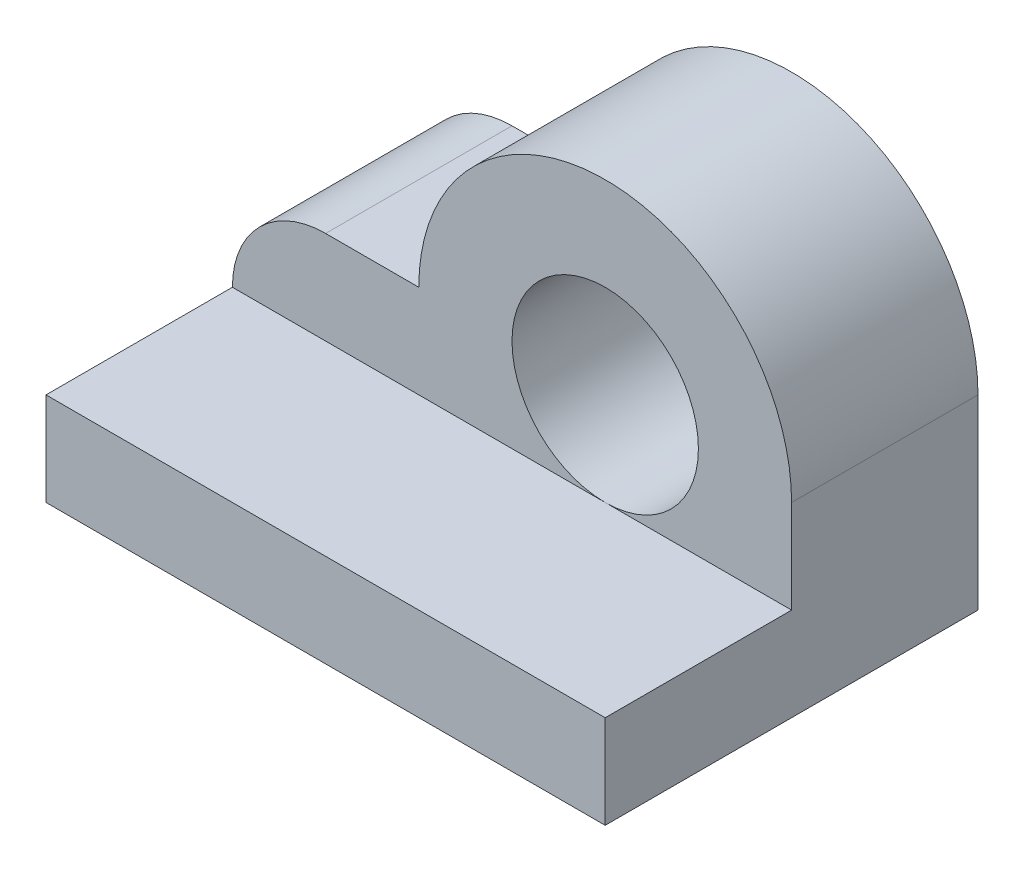
ISO-10303-21;
HEADER;
FILE_DESCRIPTION(('STEP AP214'),'2;1');
FILE_NAME('part.step','',(''),(''),'','','');
FILE_SCHEMA(('AUTOMOTIVE_DESIGN { 1 0 10303 214 1 1 1 1 }'));
ENDSEC;
DATA;
#1=APPLICATION_CONTEXT('core data for automotive mechanical design processes');
#2=APPLICATION_PROTOCOL_DEFINITION('international standard','automotive_design',2000,#1);
#3=PRODUCT_CONTEXT('',#1,'mechanical');
#4=PRODUCT('Part','Part','',(#3));
#5=PRODUCT_RELATED_PRODUCT_CATEGORY('part','',(#4));
#6=PRODUCT_DEFINITION_FORMATION('','',#4);
#7=PRODUCT_DEFINITION_CONTEXT('part definition',#1,'design');
#8=PRODUCT_DEFINITION('design','',#6,#7);
#9=PRODUCT_DEFINITION_SHAPE('','',#8);
#10=(LENGTH_UNIT() NAMED_UNIT(*) SI_UNIT(.MILLI.,.METRE.));
#11=(NAMED_UNIT(*) PLANE_ANGLE_UNIT() SI_UNIT($,.RADIAN.));
#12=(NAMED_UNIT(*) SI_UNIT($,.STERADIAN.) SOLID_ANGLE_UNIT());
#13=UNCERTAINTY_MEASURE_WITH_UNIT(LENGTH_MEASURE(1.E-05),#10,'distance_accuracy_value','');
#14=(GEOMETRIC_REPRESENTATION_CONTEXT(3) GLOBAL_UNCERTAINTY_ASSIGNED_CONTEXT((#13)) GLOBAL_UNIT_ASSIGNED_CONTEXT((#10,
#11,#12)) REPRESENTATION_CONTEXT('',''));
#15=CARTESIAN_POINT('',(0.,0.,0.));
#16=DIRECTION('',(0.,0.,1.));
#17=DIRECTION('',(1.,0.,0.));
#18=AXIS2_PLACEMENT_3D('',#15,#16,#17);
#19=CARTESIAN_POINT('',(-30.,5.,-20.));
#20=DIRECTION('',(0.,0.,1.));
#21=DIRECTION('',(1.,0.,0.));
#22=AXIS2_PLACEMENT_3D('',#19,#20,#21);
#23=PLANE('',#22);
#24=CARTESIAN_POINT('',(10.,15.,-20.));
#25=DIRECTION('',(0.,0.,-1.));
#26=DIRECTION('',(-1.,0.,0.));
#27=AXIS2_PLACEMENT_3D('',#24,#25,#26);
#28=CIRCLE('',#27,10.);
#29=CARTESIAN_POINT('',(0.,15.,-20.));
#30=VERTEX_POINT('',#29);
#31=EDGE_CURVE('E123',#30,#30,#28,.T.);
#32=ORIENTED_EDGE('',*,*,#31,.F.);
#33=EDGE_LOOP('',(#32));
#34=FACE_BOUND('',#33,.T.);
#35=DIRECTION('',(0.,-1.,0.));
#36=VECTOR('',#35,1.);
#37=CARTESIAN_POINT('',(-30.,5.,-20.));
#38=LINE('',#37,#36);
#39=CARTESIAN_POINT('',(-30.,5.,-20.));
#40=VERTEX_POINT('',#39);
#41=CARTESIAN_POINT('',(-30.,-5.,-20.));
#42=VERTEX_POINT('',#41);
#43=EDGE_CURVE('E160',#40,#42,#38,.T.);
#44=ORIENTED_EDGE('',*,*,#43,.F.);
#45=CARTESIAN_POINT('',(-20.,5.,-20.));
#46=DIRECTION('',(0.,0.,1.));
#47=DIRECTION('',(1.,0.,0.));
#48=AXIS2_PLACEMENT_3D('',#45,#46,#47);
#49=CIRCLE('',#48,10.);
#50=CARTESIAN_POINT('',(-20.,15.,-20.));
#51=VERTEX_POINT('',#50);
#52=EDGE_CURVE('E64',#40,#51,#49,.F.);
#53=ORIENTED_EDGE('',*,*,#52,.T.);
#54=DIRECTION('',(-1.,0.,0.));
#55=VECTOR('',#54,1.);
#56=CARTESIAN_POINT('',(0.,15.,-20.));
#57=LINE('',#56,#55);
#58=CARTESIAN_POINT('',(-10.,15.,-20.));
#59=VERTEX_POINT('',#58);
#60=EDGE_CURVE('E116',#59,#51,#57,.T.);
#61=ORIENTED_EDGE('',*,*,#60,.F.);
#62=CARTESIAN_POINT('',(10.,15.,-20.));
#63=DIRECTION('',(0.,0.,-1.));
#64=DIRECTION('',(-1.,0.,0.));
#65=AXIS2_PLACEMENT_3D('',#62,#63,#64);
#66=CIRCLE('',#65,20.);
#67=CARTESIAN_POINT('',(30.,15.,-20.));
#68=VERTEX_POINT('',#67);
#69=EDGE_CURVE('E106',#59,#68,#66,.T.);
#70=ORIENTED_EDGE('',*,*,#69,.T.);
#71=DIRECTION('',(0.,-1.,0.));
#72=VECTOR('',#71,1.);
#73=CARTESIAN_POINT('',(30.,5.,-20.));
#74=LINE('',#73,#72);
#75=CARTESIAN_POINT('',(30.,-5.,-20.));
#76=VERTEX_POINT('',#75);
#77=EDGE_CURVE('E157',#68,#76,#74,.T.);
#78=ORIENTED_EDGE('',*,*,#77,.T.);
#79=DIRECTION('',(-1.,0.,0.));
#80=VECTOR('',#79,1.);
#81=CARTESIAN_POINT('',(-30.,-5.,-20.));
#82=LINE('',#81,#80);
#83=EDGE_CURVE('E148',#76,#42,#82,.T.);
#84=ORIENTED_EDGE('',*,*,#83,.T.);
#85=EDGE_LOOP('',(#44,#53,#61,#70,#78,#84));
#86=FACE_BOUND('',#85,.T.);
#87=ADVANCED_FACE('F41',(#34,#86),#23,.F.);
#88=CARTESIAN_POINT('',(-30.,35.,0.));
#89=DIRECTION('',(0.,0.,-1.));
#90=DIRECTION('',(-1.,0.,0.));
#91=AXIS2_PLACEMENT_3D('',#88,#89,#90);
#92=PLANE('',#91);
#93=DIRECTION('',(-1.,0.,0.));
#94=VECTOR('',#93,1.);
#95=CARTESIAN_POINT('',(-30.,15.,0.));
#96=LINE('',#95,#94);
#97=CARTESIAN_POINT('',(-10.,15.,0.));
#98=VERTEX_POINT('',#97);
#99=CARTESIAN_POINT('',(-20.,15.,0.));
#100=VERTEX_POINT('',#99);
#101=EDGE_CURVE('E114',#98,#100,#96,.T.);
#102=ORIENTED_EDGE('',*,*,#101,.T.);
#103=CARTESIAN_POINT('',(-20.,5.,0.));
#104=DIRECTION('',(0.,0.,-1.));
#105=DIRECTION('',(-1.,0.,0.));
#106=AXIS2_PLACEMENT_3D('',#103,#104,#105);
#107=CIRCLE('',#106,10.);
#108=CARTESIAN_POINT('',(-30.,5.,0.));
#109=VERTEX_POINT('',#108);
#110=EDGE_CURVE('E11',#100,#109,#107,.F.);
#111=ORIENTED_EDGE('',*,*,#110,.T.);
#112=DIRECTION('',(1.,0.,0.));
#113=VECTOR('',#112,1.);
#114=CARTESIAN_POINT('',(-30.,5.,0.));
#115=LINE('',#114,#113);
#116=CARTESIAN_POINT('',(10.,5.,0.));
#117=VERTEX_POINT('',#116);
#118=EDGE_CURVE('E126',#109,#117,#115,.T.);
#119=ORIENTED_EDGE('',*,*,#118,.T.);
#120=CARTESIAN_POINT('',(10.,15.,0.));
#121=DIRECTION('',(0.,0.,-1.));
#122=DIRECTION('',(-1.,0.,0.));
#123=AXIS2_PLACEMENT_3D('',#120,#121,#122);
#124=CIRCLE('',#123,10.);
#125=EDGE_CURVE('E130',#117,#117,#124,.T.);
#126=ORIENTED_EDGE('',*,*,#125,.T.);
#127=CARTESIAN_POINT('',(30.,5.,0.));
#128=VERTEX_POINT('',#127);
#129=EDGE_CURVE('E132',#117,#128,#115,.T.);
#130=ORIENTED_EDGE('',*,*,#129,.T.);
#131=DIRECTION('',(0.,-1.,0.));
#132=VECTOR('',#131,1.);
#133=CARTESIAN_POINT('',(30.,35.,0.));
#134=LINE('',#133,#132);
#135=CARTESIAN_POINT('',(30.,15.,0.));
#136=VERTEX_POINT('',#135);
#137=EDGE_CURVE('E131',#136,#128,#134,.T.);
#138=ORIENTED_EDGE('',*,*,#137,.F.);
#139=CARTESIAN_POINT('',(10.,15.,0.));
#140=DIRECTION('',(0.,0.,-1.));
#141=DIRECTION('',(-1.,0.,0.));
#142=AXIS2_PLACEMENT_3D('',#139,#140,#141);
#143=CIRCLE('',#142,20.);
#144=EDGE_CURVE('E122',#98,#136,#143,.T.);
#145=ORIENTED_EDGE('',*,*,#144,.F.);
#146=EDGE_LOOP('',(#102,#111,#119,#126,#130,#138,#145));
#147=FACE_BOUND('',#146,.T.);
#148=ADVANCED_FACE('F190',(#147),#92,.F.);
#149=CARTESIAN_POINT('',(30.,5.,20.));
#150=DIRECTION('',(-1.,0.,0.));
#151=DIRECTION('',(0.,0.,1.));
#152=AXIS2_PLACEMENT_3D('',#149,#150,#151);
#153=PLANE('',#152);
#154=DIRECTION('',(0.,0.,-1.));
#155=VECTOR('',#154,1.);
#156=CARTESIAN_POINT('',(30.,15.,20.));
#157=LINE('',#156,#155);
#158=EDGE_CURVE('E112',#136,#68,#157,.T.);
#159=ORIENTED_EDGE('',*,*,#158,.F.);
#160=ORIENTED_EDGE('',*,*,#137,.T.);
#161=DIRECTION('',(0.,0.,-1.));
#162=VECTOR('',#161,1.);
#163=CARTESIAN_POINT('',(30.,5.,20.));
#164=LINE('',#163,#162);
#165=CARTESIAN_POINT('',(30.,5.,20.));
#166=VERTEX_POINT('',#165);
#167=EDGE_CURVE('E135',#166,#128,#164,.T.);
#168=ORIENTED_EDGE('',*,*,#167,.F.);
#169=DIRECTION('',(0.,-1.,0.));
#170=VECTOR('',#169,1.);
#171=CARTESIAN_POINT('',(30.,5.,20.));
#172=LINE('',#171,#170);
#173=CARTESIAN_POINT('',(30.,-5.,20.));
#174=VERTEX_POINT('',#173);
#175=EDGE_CURVE('E141',#166,#174,#172,.T.);
#176=ORIENTED_EDGE('',*,*,#175,.T.);
#177=DIRECTION('',(0.,0.,-1.));
#178=VECTOR('',#177,1.);
#179=CARTESIAN_POINT('',(30.,-5.,20.));
#180=LINE('',#179,#178);
#181=EDGE_CURVE('E133',#174,#76,#180,.T.);
#182=ORIENTED_EDGE('',*,*,#181,.T.);
#183=ORIENTED_EDGE('',*,*,#77,.F.);
#184=EDGE_LOOP('',(#159,#160,#168,#176,#182,#183));
#185=FACE_BOUND('',#184,.T.);
#186=ADVANCED_FACE('F201',(#185),#153,.F.);
#187=CARTESIAN_POINT('',(0.,5.,0.));
#188=DIRECTION('',(0.,-1.,0.));
#189=DIRECTION('',(0.,0.,-1.));
#190=AXIS2_PLACEMENT_3D('',#187,#188,#189);
#191=PLANE('',#190);
#192=DIRECTION('',(1.,0.,0.));
#193=VECTOR('',#192,1.);
#194=CARTESIAN_POINT('',(-30.,5.,20.));
#195=LINE('',#194,#193);
#196=CARTESIAN_POINT('',(-30.,5.,20.));
#197=VERTEX_POINT('',#196);
#198=EDGE_CURVE('E143',#197,#166,#195,.T.);
#199=ORIENTED_EDGE('',*,*,#198,.T.);
#200=ORIENTED_EDGE('',*,*,#167,.T.);
#201=ORIENTED_EDGE('',*,*,#129,.F.);
#202=ORIENTED_EDGE('',*,*,#118,.F.);
#203=DIRECTION('',(0.,0.,1.));
#204=VECTOR('',#203,1.);
#205=CARTESIAN_POINT('',(-30.,5.,20.));
#206=LINE('',#205,#204);
#207=EDGE_CURVE('E139',#109,#197,#206,.T.);
#208=ORIENTED_EDGE('',*,*,#207,.T.);
#209=EDGE_LOOP('',(#199,#200,#201,#202,#208));
#210=FACE_BOUND('',#209,.T.);
#211=ADVANCED_FACE('F183',(#210),#191,.F.);
#212=CARTESIAN_POINT('',(-30.,5.,20.));
#213=DIRECTION('',(1.,0.,0.));
#214=DIRECTION('',(0.,0.,-1.));
#215=AXIS2_PLACEMENT_3D('',#212,#213,#214);
#216=PLANE('',#215);
#217=ORIENTED_EDGE('',*,*,#207,.F.);
#218=DIRECTION('',(0.,0.,-1.));
#219=VECTOR('',#218,1.);
#220=CARTESIAN_POINT('',(-30.,5.,20.));
#221=LINE('',#220,#219);
#222=EDGE_CURVE('E161',#109,#40,#221,.T.);
#223=ORIENTED_EDGE('',*,*,#222,.T.);
#224=ORIENTED_EDGE('',*,*,#43,.T.);
#225=DIRECTION('',(0.,0.,1.));
#226=VECTOR('',#225,1.);
#227=CARTESIAN_POINT('',(-30.,-5.,20.));
#228=LINE('',#227,#226);
#229=CARTESIAN_POINT('',(-30.,-5.,20.));
#230=VERTEX_POINT('',#229);
#231=EDGE_CURVE('E149',#42,#230,#228,.T.);
#232=ORIENTED_EDGE('',*,*,#231,.T.);
#233=DIRECTION('',(0.,-1.,0.));
#234=VECTOR('',#233,1.);
#235=CARTESIAN_POINT('',(-30.,5.,20.));
#236=LINE('',#235,#234);
#237=EDGE_CURVE('E152',#197,#230,#236,.T.);
#238=ORIENTED_EDGE('',*,*,#237,.F.);
#239=EDGE_LOOP('',(#217,#223,#224,#232,#238));
#240=FACE_BOUND('',#239,.T.);
#241=ADVANCED_FACE('F166',(#240),#216,.F.);
#242=CARTESIAN_POINT('',(-30.,5.,20.));
#243=DIRECTION('',(0.,0.,-1.));
#244=DIRECTION('',(-1.,0.,0.));
#245=AXIS2_PLACEMENT_3D('',#242,#243,#244);
#246=PLANE('',#245);
#247=DIRECTION('',(1.,0.,0.));
#248=VECTOR('',#247,1.);
#249=CARTESIAN_POINT('',(-30.,-5.,20.));
#250=LINE('',#249,#248);
#251=EDGE_CURVE('E138',#230,#174,#250,.T.);
#252=ORIENTED_EDGE('',*,*,#251,.T.);
#253=ORIENTED_EDGE('',*,*,#175,.F.);
#254=ORIENTED_EDGE('',*,*,#198,.F.);
#255=ORIENTED_EDGE('',*,*,#237,.T.);
#256=EDGE_LOOP('',(#252,#253,#254,#255));
#257=FACE_BOUND('',#256,.T.);
#258=ADVANCED_FACE('F182',(#257),#246,.F.);
#259=CARTESIAN_POINT('',(0.,-5.,0.));
#260=DIRECTION('',(0.,-1.,0.));
#261=DIRECTION('',(0.,0.,-1.));
#262=AXIS2_PLACEMENT_3D('',#259,#260,#261);
#263=PLANE('',#262);
#264=ORIENTED_EDGE('',*,*,#181,.F.);
#265=ORIENTED_EDGE('',*,*,#251,.F.);
#266=ORIENTED_EDGE('',*,*,#231,.F.);
#267=ORIENTED_EDGE('',*,*,#83,.F.);
#268=EDGE_LOOP('',(#264,#265,#266,#267));
#269=FACE_BOUND('',#268,.T.);
#270=ADVANCED_FACE('F179',(#269),#263,.T.);
#271=CARTESIAN_POINT('',(10.,15.,20.));
#272=DIRECTION('',(0.,0.,-1.));
#273=DIRECTION('',(-1.,0.,0.));
#274=AXIS2_PLACEMENT_3D('',#271,#272,#273);
#275=CYLINDRICAL_SURFACE('',#274,10.);
#276=ORIENTED_EDGE('',*,*,#31,.T.);
#277=EDGE_LOOP('',(#276));
#278=FACE_BOUND('',#277,.T.);
#279=ORIENTED_EDGE('',*,*,#125,.F.);
#280=EDGE_LOOP('',(#279));
#281=FACE_BOUND('',#280,.T.);
#282=ADVANCED_FACE('F225',(#278,#281),#275,.F.);
#283=CARTESIAN_POINT('',(10.,15.,20.));
#284=DIRECTION('',(0.,0.,-1.));
#285=DIRECTION('',(-1.,0.,0.));
#286=AXIS2_PLACEMENT_3D('',#283,#284,#285);
#287=CYLINDRICAL_SURFACE('',#286,20.);
#288=ORIENTED_EDGE('',*,*,#144,.T.);
#289=ORIENTED_EDGE('',*,*,#158,.T.);
#290=ORIENTED_EDGE('',*,*,#69,.F.);
#291=DIRECTION('',(0.,0.,-1.));
#292=VECTOR('',#291,1.);
#293=CARTESIAN_POINT('',(-10.,15.,20.));
#294=LINE('',#293,#292);
#295=EDGE_CURVE('E108',#98,#59,#294,.T.);
#296=ORIENTED_EDGE('',*,*,#295,.F.);
#297=EDGE_LOOP('',(#288,#289,#290,#296));
#298=FACE_BOUND('',#297,.T.);
#299=ADVANCED_FACE('F107',(#298),#287,.T.);
#300=CARTESIAN_POINT('',(0.,15.,20.));
#301=DIRECTION('',(0.,-1.,0.));
#302=DIRECTION('',(0.,0.,-1.));
#303=AXIS2_PLACEMENT_3D('',#300,#301,#302);
#304=PLANE('',#303);
#305=ORIENTED_EDGE('',*,*,#60,.T.);
#306=DIRECTION('',(0.,0.,-1.));
#307=VECTOR('',#306,1.);
#308=CARTESIAN_POINT('',(-20.,15.,20.));
#309=LINE('',#308,#307);
#310=EDGE_CURVE('E47',#51,#100,#309,.F.);
#311=ORIENTED_EDGE('',*,*,#310,.T.);
#312=ORIENTED_EDGE('',*,*,#101,.F.);
#313=ORIENTED_EDGE('',*,*,#295,.T.);
#314=EDGE_LOOP('',(#305,#311,#312,#313));
#315=FACE_BOUND('',#314,.T.);
#316=ADVANCED_FACE('F113',(#315),#304,.F.);
#317=CARTESIAN_POINT('',(-20.,5.,20.));
#318=DIRECTION('',(0.,0.,-1.));
#319=DIRECTION('',(-1.,0.,0.));
#320=AXIS2_PLACEMENT_3D('',#317,#318,#319);
#321=CYLINDRICAL_SURFACE('',#320,10.);
#322=ORIENTED_EDGE('',*,*,#110,.F.);
#323=ORIENTED_EDGE('',*,*,#310,.F.);
#324=ORIENTED_EDGE('',*,*,#52,.F.);
#325=ORIENTED_EDGE('',*,*,#222,.F.);
#326=EDGE_LOOP('',(#322,#323,#324,#325));
#327=FACE_BOUND('',#326,.T.);
#328=ADVANCED_FACE('F43',(#327),#321,.T.);
#329=CLOSED_SHELL('',(#87,#148,#186,#211,#241,#258,#270,#282,#299,#316,#328));
#330=MANIFOLD_SOLID_BREP('B2',#329);
#331=ADVANCED_BREP_SHAPE_REPRESENTATION('',(#18,#330),#14);
#332=SHAPE_DEFINITION_REPRESENTATION(#9,#331);
ENDSEC;
END-ISO-10303-21;
